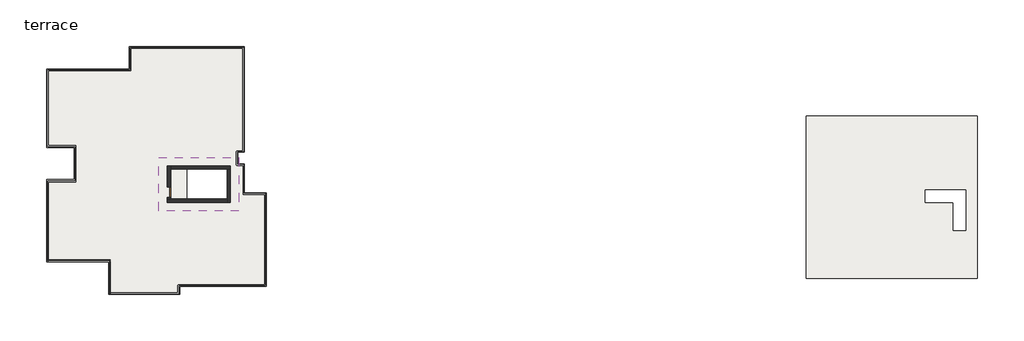
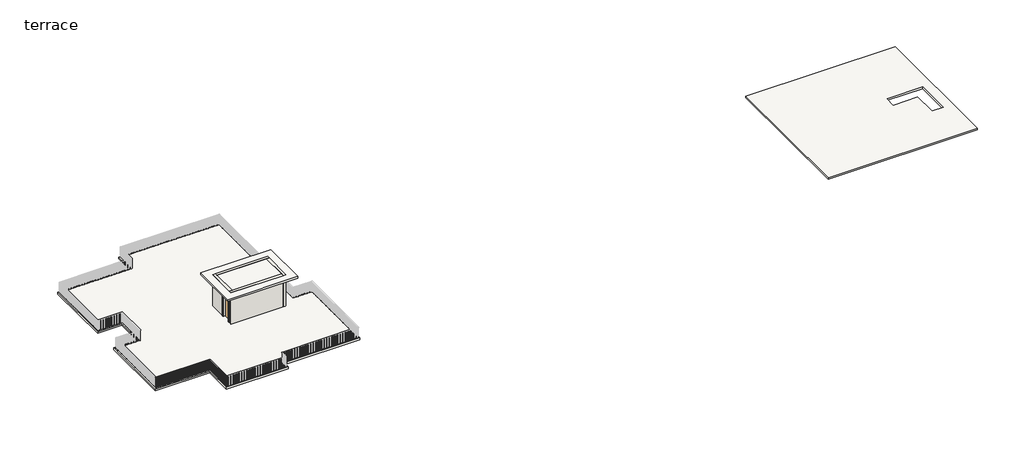
# One storey, part 1 of 7: 4 walls, 3 slabs, 2 railings, 1 door.
"""IFC4 building model written with IfcOpenShell, lengths in millimetres."""

from ifc_helpers import new_model, si_unit, frame, origin, place, context, project, spatial, polyline, outline, extrude, faceted_brep, transform, mapped, element, save
from components import door_bb98abfd

model = new_model("IFC4")

# Units and contexts
model_context = context("Model", 3, world=origin())
ifc_project = project(units=[si_unit("LENGTHUNIT", "METRE", prefix="MILLI")], contexts=[model_context])

# Site, building, storey
site = spatial("IfcSite", under=ifc_project)
building = spatial("IfcBuilding", under=site)
storey = spatial("IfcBuildingStorey", under=building, Name="terrace", Elevation=3810.0)

# Door
placement = place(None, origin())
door_shape = door_bb98abfd(model_context)
element("IfcDoor", 1, ObjectType="Single-Flush : 30\" x 84\"", at=placement, inside=storey, context=model_context, shape_type="MappedRepresentation", body=[
    mapped(door_shape, transform((-5641.4918815, 2189.5168074, 3810.0), x_axis=(0.0, -1.0, 0.0), y_axis=(1.0, 0.0, 0.0), z_axis=(0.0, 0.0, 1.0))),
])

# Railings
element("IfcRailing", 2, ObjectType="Handrail - Rectangular", at=placement, inside=storey, context=model_context, shape_type="SweptSolid", body=[
    extrude(outline(polyline([(-9876.7390129, -5140.022378), (-9927.5390129, -5140.022378), (-9927.5390129, -2803.222378), (-9876.7390129, -2803.222378), (-9876.7390129, -5140.022378)])), frame((0.0, 0.0, 4673.6), z_axis=(0.0, 0.0, 1.0), x_axis=(1.0, 0.0, 0.0)), (0.0, 0.0, 1.0), 50.8),
    extrude(outline(polyline([(-9892.6140129, -2914.347378), (-9911.6640129, -2914.347378), (-9911.6640129, -2895.297378), (-9892.6140129, -2895.297378), (-9892.6140129, -2914.347378)])), frame((0.0, 0.0, 3810.0), z_axis=(0.0, 0.0, 1.0), x_axis=(1.0, 0.0, 0.0)), (0.0, 0.0, 1.0), 863.6),
    extrude(outline(polyline([(-9892.6140129, -3015.947378), (-9911.6640129, -3015.947378), (-9911.6640129, -2996.897378), (-9892.6140129, -2996.897378), (-9892.6140129, -3015.947378)])), frame((0.0, 0.0, 3810.0), z_axis=(0.0, 0.0, 1.0), x_axis=(1.0, 0.0, 0.0)), (0.0, 0.0, 1.0), 863.6),
    extrude(outline(polyline([(-9892.6140129, -3117.547378), (-9911.6640129, -3117.547378), (-9911.6640129, -3098.497378), (-9892.6140129, -3098.497378), (-9892.6140129, -3117.547378)])), frame((0.0, 0.0, 3810.0), z_axis=(0.0, 0.0, 1.0), x_axis=(1.0, 0.0, 0.0)), (0.0, 0.0, 1.0), 863.6),
    extrude(outline(polyline([(-9892.6140129, -3219.147378), (-9911.6640129, -3219.147378), (-9911.6640129, -3200.097378), (-9892.6140129, -3200.097378), (-9892.6140129, -3219.147378)])), frame((0.0, 0.0, 3810.0), z_axis=(0.0, 0.0, 1.0), x_axis=(1.0, 0.0, 0.0)), (0.0, 0.0, 1.0), 863.6),
    extrude(outline(polyline([(-9892.6140129, -3320.747378), (-9911.6640129, -3320.747378), (-9911.6640129, -3301.697378), (-9892.6140129, -3301.697378), (-9892.6140129, -3320.747378)])), frame((0.0, 0.0, 3810.0), z_axis=(0.0, 0.0, 1.0), x_axis=(1.0, 0.0, 0.0)), (0.0, 0.0, 1.0), 863.6),
    extrude(outline(polyline([(-9892.6140129, -3422.347378), (-9911.6640129, -3422.347378), (-9911.6640129, -3403.297378), (-9892.6140129, -3403.297378), (-9892.6140129, -3422.347378)])), frame((0.0, 0.0, 3810.0), z_axis=(0.0, 0.0, 1.0), x_axis=(1.0, 0.0, 0.0)), (0.0, 0.0, 1.0), 863.6),
    extrude(outline(polyline([(-9892.6140129, -3523.947378), (-9911.6640129, -3523.947378), (-9911.6640129, -3504.897378), (-9892.6140129, -3504.897378), (-9892.6140129, -3523.947378)])), frame((0.0, 0.0, 3810.0), z_axis=(0.0, 0.0, 1.0), x_axis=(1.0, 0.0, 0.0)), (0.0, 0.0, 1.0), 863.6),
    extrude(outline(polyline([(-9892.6140129, -3625.547378), (-9911.6640129, -3625.547378), (-9911.6640129, -3606.497378), (-9892.6140129, -3606.497378), (-9892.6140129, -3625.547378)])), frame((0.0, 0.0, 3810.0), z_axis=(0.0, 0.0, 1.0), x_axis=(1.0, 0.0, 0.0)), (0.0, 0.0, 1.0), 863.6),
    extrude(outline(polyline([(-9892.6140129, -3727.147378), (-9911.6640129, -3727.147378), (-9911.6640129, -3708.097378), (-9892.6140129, -3708.097378), (-9892.6140129, -3727.147378)])), frame((0.0, 0.0, 3810.0), z_axis=(0.0, 0.0, 1.0), x_axis=(1.0, 0.0, 0.0)), (0.0, 0.0, 1.0), 863.6),
    extrude(outline(polyline([(-9892.6140129, -3828.747378), (-9911.6640129, -3828.747378), (-9911.6640129, -3809.697378), (-9892.6140129, -3809.697378), (-9892.6140129, -3828.747378)])), frame((0.0, 0.0, 3810.0), z_axis=(0.0, 0.0, 1.0), x_axis=(1.0, 0.0, 0.0)), (0.0, 0.0, 1.0), 863.6),
    extrude(outline(polyline([(-9892.6140129, -3930.347378), (-9911.6640129, -3930.347378), (-9911.6640129, -3911.297378), (-9892.6140129, -3911.297378), (-9892.6140129, -3930.347378)])), frame((0.0, 0.0, 3810.0), z_axis=(0.0, 0.0, 1.0), x_axis=(1.0, 0.0, 0.0)), (0.0, 0.0, 1.0), 863.6),
    extrude(outline(polyline([(-9892.6140129, -4031.947378), (-9911.6640129, -4031.947378), (-9911.6640129, -4012.897378), (-9892.6140129, -4012.897378), (-9892.6140129, -4031.947378)])), frame((0.0, 0.0, 3810.0), z_axis=(0.0, 0.0, 1.0), x_axis=(1.0, 0.0, 0.0)), (0.0, 0.0, 1.0), 863.6),
    extrude(outline(polyline([(-9892.6140129, -4133.547378), (-9911.6640129, -4133.547378), (-9911.6640129, -4114.497378), (-9892.6140129, -4114.497378), (-9892.6140129, -4133.547378)])), frame((0.0, 0.0, 3810.0), z_axis=(0.0, 0.0, 1.0), x_axis=(1.0, 0.0, 0.0)), (0.0, 0.0, 1.0), 863.6),
    extrude(outline(polyline([(-9892.6140129, -4235.147378), (-9911.6640129, -4235.147378), (-9911.6640129, -4216.097378), (-9892.6140129, -4216.097378), (-9892.6140129, -4235.147378)])), frame((0.0, 0.0, 3810.0), z_axis=(0.0, 0.0, 1.0), x_axis=(1.0, 0.0, 0.0)), (0.0, 0.0, 1.0), 863.6),
    extrude(outline(polyline([(-9892.6140129, -4336.747378), (-9911.6640129, -4336.747378), (-9911.6640129, -4317.697378), (-9892.6140129, -4317.697378), (-9892.6140129, -4336.747378)])), frame((0.0, 0.0, 3810.0), z_axis=(0.0, 0.0, 1.0), x_axis=(1.0, 0.0, 0.0)), (0.0, 0.0, 1.0), 863.6),
    extrude(outline(polyline([(-9892.6140129, -4438.347378), (-9911.6640129, -4438.347378), (-9911.6640129, -4419.297378), (-9892.6140129, -4419.297378), (-9892.6140129, -4438.347378)])), frame((0.0, 0.0, 3810.0), z_axis=(0.0, 0.0, 1.0), x_axis=(1.0, 0.0, 0.0)), (0.0, 0.0, 1.0), 863.6),
    extrude(outline(polyline([(-9892.6140129, -4539.947378), (-9911.6640129, -4539.947378), (-9911.6640129, -4520.897378), (-9892.6140129, -4520.897378), (-9892.6140129, -4539.947378)])), frame((0.0, 0.0, 3810.0), z_axis=(0.0, 0.0, 1.0), x_axis=(1.0, 0.0, 0.0)), (0.0, 0.0, 1.0), 863.6),
    extrude(outline(polyline([(-9892.6140129, -4641.547378), (-9911.6640129, -4641.547378), (-9911.6640129, -4622.497378), (-9892.6140129, -4622.497378), (-9892.6140129, -4641.547378)])), frame((0.0, 0.0, 3810.0), z_axis=(0.0, 0.0, 1.0), x_axis=(1.0, 0.0, 0.0)), (0.0, 0.0, 1.0), 863.6),
    extrude(outline(polyline([(-9892.6140129, -4743.147378), (-9911.6640129, -4743.147378), (-9911.6640129, -4724.097378), (-9892.6140129, -4724.097378), (-9892.6140129, -4743.147378)])), frame((0.0, 0.0, 3810.0), z_axis=(0.0, 0.0, 1.0), x_axis=(1.0, 0.0, 0.0)), (0.0, 0.0, 1.0), 863.6),
    extrude(outline(polyline([(-9892.6140129, -4844.747378), (-9911.6640129, -4844.747378), (-9911.6640129, -4825.697378), (-9892.6140129, -4825.697378), (-9892.6140129, -4844.747378)])), frame((0.0, 0.0, 3810.0), z_axis=(0.0, 0.0, 1.0), x_axis=(1.0, 0.0, 0.0)), (0.0, 0.0, 1.0), 863.6),
    extrude(outline(polyline([(-9892.6140129, -4946.347378), (-9911.6640129, -4946.347378), (-9911.6640129, -4927.297378), (-9892.6140129, -4927.297378), (-9892.6140129, -4946.347378)])), frame((0.0, 0.0, 3810.0), z_axis=(0.0, 0.0, 1.0), x_axis=(1.0, 0.0, 0.0)), (0.0, 0.0, 1.0), 863.6),
    extrude(outline(polyline([(-9892.6140129, -5047.947378), (-9911.6640129, -5047.947378), (-9911.6640129, -5028.897378), (-9892.6140129, -5028.897378), (-9892.6140129, -5047.947378)])), frame((0.0, 0.0, 3810.0), z_axis=(0.0, 0.0, 1.0), x_axis=(1.0, 0.0, 0.0)), (0.0, 0.0, 1.0), 863.6),
    extrude(outline(polyline([(-9892.6140129, -2822.272378), (-9911.6640129, -2822.272378), (-9911.6640129, -2803.222378), (-9892.6140129, -2803.222378), (-9892.6140129, -2822.272378)])), frame((0.0, 0.0, 3810.0), z_axis=(0.0, 0.0, 1.0), x_axis=(1.0, 0.0, 0.0)), (0.0, 0.0, 1.0), 863.6),
    extrude(outline(polyline([(-9892.6140129, -5140.022378), (-9911.6640129, -5140.022378), (-9911.6640129, -5120.972378), (-9892.6140129, -5120.972378), (-9892.6140129, -5140.022378)])), frame((0.0, 0.0, 3810.0), z_axis=(0.0, 0.0, 1.0), x_axis=(1.0, 0.0, 0.0)), (0.0, 0.0, 1.0), 863.6),
])
element("IfcRailing", 3, ObjectType="Handrail - Rectangular", at=placement, inside=storey, context=model_context, shape_type="SweptSolid", body=[
    extrude(outline(polyline([(-9895.7890129, -2701.622378), (-9895.7890129, -2752.422378), (-14391.5890129, -2752.422378), (-14391.5890129, -2701.622378), (-9895.7890129, -2701.622378)])), frame((0.0, 0.0, 4673.6), z_axis=(0.0, 0.0, 1.0), x_axis=(1.0, 0.0, 0.0)), (0.0, 0.0, 1.0), 50.8),
    extrude(outline(polyline([(-14356.6640129, -2717.497378), (-14356.6640129, -2736.547378), (-14375.7140129, -2736.547378), (-14375.7140129, -2717.497378), (-14356.6640129, -2717.497378)])), frame((0.0, 0.0, 3810.0), z_axis=(0.0, 0.0, 1.0), x_axis=(1.0, 0.0, 0.0)), (0.0, 0.0, 1.0), 863.6),
    extrude(outline(polyline([(-14255.0640129, -2717.497378), (-14255.0640129, -2736.547378), (-14274.1140129, -2736.547378), (-14274.1140129, -2717.497378), (-14255.0640129, -2717.497378)])), frame((0.0, 0.0, 3810.0), z_axis=(0.0, 0.0, 1.0), x_axis=(1.0, 0.0, 0.0)), (0.0, 0.0, 1.0), 863.6),
    extrude(outline(polyline([(-14153.4640129, -2717.497378), (-14153.4640129, -2736.547378), (-14172.5140129, -2736.547378), (-14172.5140129, -2717.497378), (-14153.4640129, -2717.497378)])), frame((0.0, 0.0, 3810.0), z_axis=(0.0, 0.0, 1.0), x_axis=(1.0, 0.0, 0.0)), (0.0, 0.0, 1.0), 863.6),
    extrude(outline(polyline([(-14051.8640129, -2717.497378), (-14051.8640129, -2736.547378), (-14070.9140129, -2736.547378), (-14070.9140129, -2717.497378), (-14051.8640129, -2717.497378)])), frame((0.0, 0.0, 3810.0), z_axis=(0.0, 0.0, 1.0), x_axis=(1.0, 0.0, 0.0)), (0.0, 0.0, 1.0), 863.6),
    extrude(outline(polyline([(-13950.2640129, -2717.497378), (-13950.2640129, -2736.547378), (-13969.3140129, -2736.547378), (-13969.3140129, -2717.497378), (-13950.2640129, -2717.497378)])), frame((0.0, 0.0, 3810.0), z_axis=(0.0, 0.0, 1.0), x_axis=(1.0, 0.0, 0.0)), (0.0, 0.0, 1.0), 863.6),
    extrude(outline(polyline([(-13848.6640129, -2717.497378), (-13848.6640129, -2736.547378), (-13867.7140129, -2736.547378), (-13867.7140129, -2717.497378), (-13848.6640129, -2717.497378)])), frame((0.0, 0.0, 3810.0), z_axis=(0.0, 0.0, 1.0), x_axis=(1.0, 0.0, 0.0)), (0.0, 0.0, 1.0), 863.6),
    extrude(outline(polyline([(-13747.0640129, -2717.497378), (-13747.0640129, -2736.547378), (-13766.1140129, -2736.547378), (-13766.1140129, -2717.497378), (-13747.0640129, -2717.497378)])), frame((0.0, 0.0, 3810.0), z_axis=(0.0, 0.0, 1.0), x_axis=(1.0, 0.0, 0.0)), (0.0, 0.0, 1.0), 863.6),
    extrude(outline(polyline([(-13645.4640129, -2717.497378), (-13645.4640129, -2736.547378), (-13664.5140129, -2736.547378), (-13664.5140129, -2717.497378), (-13645.4640129, -2717.497378)])), frame((0.0, 0.0, 3810.0), z_axis=(0.0, 0.0, 1.0), x_axis=(1.0, 0.0, 0.0)), (0.0, 0.0, 1.0), 863.6),
    extrude(outline(polyline([(-13543.8640129, -2717.497378), (-13543.8640129, -2736.547378), (-13562.9140129, -2736.547378), (-13562.9140129, -2717.497378), (-13543.8640129, -2717.497378)])), frame((0.0, 0.0, 3810.0), z_axis=(0.0, 0.0, 1.0), x_axis=(1.0, 0.0, 0.0)), (0.0, 0.0, 1.0), 863.6),
    extrude(outline(polyline([(-13442.2640129, -2717.497378), (-13442.2640129, -2736.547378), (-13461.3140129, -2736.547378), (-13461.3140129, -2717.497378), (-13442.2640129, -2717.497378)])), frame((0.0, 0.0, 3810.0), z_axis=(0.0, 0.0, 1.0), x_axis=(1.0, 0.0, 0.0)), (0.0, 0.0, 1.0), 863.6),
    extrude(outline(polyline([(-13340.6640129, -2717.497378), (-13340.6640129, -2736.547378), (-13359.7140129, -2736.547378), (-13359.7140129, -2717.497378), (-13340.6640129, -2717.497378)])), frame((0.0, 0.0, 3810.0), z_axis=(0.0, 0.0, 1.0), x_axis=(1.0, 0.0, 0.0)), (0.0, 0.0, 1.0), 863.6),
    extrude(outline(polyline([(-13239.0640129, -2717.497378), (-13239.0640129, -2736.547378), (-13258.1140129, -2736.547378), (-13258.1140129, -2717.497378), (-13239.0640129, -2717.497378)])), frame((0.0, 0.0, 3810.0), z_axis=(0.0, 0.0, 1.0), x_axis=(1.0, 0.0, 0.0)), (0.0, 0.0, 1.0), 863.6),
    extrude(outline(polyline([(-13137.4640129, -2717.497378), (-13137.4640129, -2736.547378), (-13156.5140129, -2736.547378), (-13156.5140129, -2717.497378), (-13137.4640129, -2717.497378)])), frame((0.0, 0.0, 3810.0), z_axis=(0.0, 0.0, 1.0), x_axis=(1.0, 0.0, 0.0)), (0.0, 0.0, 1.0), 863.6),
    extrude(outline(polyline([(-13035.8640129, -2717.497378), (-13035.8640129, -2736.547378), (-13054.9140129, -2736.547378), (-13054.9140129, -2717.497378), (-13035.8640129, -2717.497378)])), frame((0.0, 0.0, 3810.0), z_axis=(0.0, 0.0, 1.0), x_axis=(1.0, 0.0, 0.0)), (0.0, 0.0, 1.0), 863.6),
    extrude(outline(polyline([(-12934.2640129, -2717.497378), (-12934.2640129, -2736.547378), (-12953.3140129, -2736.547378), (-12953.3140129, -2717.497378), (-12934.2640129, -2717.497378)])), frame((0.0, 0.0, 3810.0), z_axis=(0.0, 0.0, 1.0), x_axis=(1.0, 0.0, 0.0)), (0.0, 0.0, 1.0), 863.6),
    extrude(outline(polyline([(-12832.6640129, -2717.497378), (-12832.6640129, -2736.547378), (-12851.7140129, -2736.547378), (-12851.7140129, -2717.497378), (-12832.6640129, -2717.497378)])), frame((0.0, 0.0, 3810.0), z_axis=(0.0, 0.0, 1.0), x_axis=(1.0, 0.0, 0.0)), (0.0, 0.0, 1.0), 863.6),
    extrude(outline(polyline([(-12731.0640129, -2717.497378), (-12731.0640129, -2736.547378), (-12750.1140129, -2736.547378), (-12750.1140129, -2717.497378), (-12731.0640129, -2717.497378)])), frame((0.0, 0.0, 3810.0), z_axis=(0.0, 0.0, 1.0), x_axis=(1.0, 0.0, 0.0)), (0.0, 0.0, 1.0), 863.6),
    extrude(outline(polyline([(-12629.4640129, -2717.497378), (-12629.4640129, -2736.547378), (-12648.5140129, -2736.547378), (-12648.5140129, -2717.497378), (-12629.4640129, -2717.497378)])), frame((0.0, 0.0, 3810.0), z_axis=(0.0, 0.0, 1.0), x_axis=(1.0, 0.0, 0.0)), (0.0, 0.0, 1.0), 863.6),
    extrude(outline(polyline([(-12527.8640129, -2717.497378), (-12527.8640129, -2736.547378), (-12546.9140129, -2736.547378), (-12546.9140129, -2717.497378), (-12527.8640129, -2717.497378)])), frame((0.0, 0.0, 3810.0), z_axis=(0.0, 0.0, 1.0), x_axis=(1.0, 0.0, 0.0)), (0.0, 0.0, 1.0), 863.6),
    extrude(outline(polyline([(-12426.2640129, -2717.497378), (-12426.2640129, -2736.547378), (-12445.3140129, -2736.547378), (-12445.3140129, -2717.497378), (-12426.2640129, -2717.497378)])), frame((0.0, 0.0, 3810.0), z_axis=(0.0, 0.0, 1.0), x_axis=(1.0, 0.0, 0.0)), (0.0, 0.0, 1.0), 863.6),
    extrude(outline(polyline([(-12324.6640129, -2717.497378), (-12324.6640129, -2736.547378), (-12343.7140129, -2736.547378), (-12343.7140129, -2717.497378), (-12324.6640129, -2717.497378)])), frame((0.0, 0.0, 3810.0), z_axis=(0.0, 0.0, 1.0), x_axis=(1.0, 0.0, 0.0)), (0.0, 0.0, 1.0), 863.6),
    extrude(outline(polyline([(-12223.0640129, -2717.497378), (-12223.0640129, -2736.547378), (-12242.1140129, -2736.547378), (-12242.1140129, -2717.497378), (-12223.0640129, -2717.497378)])), frame((0.0, 0.0, 3810.0), z_axis=(0.0, 0.0, 1.0), x_axis=(1.0, 0.0, 0.0)), (0.0, 0.0, 1.0), 863.6),
    extrude(outline(polyline([(-12121.4640129, -2717.497378), (-12121.4640129, -2736.547378), (-12140.5140129, -2736.547378), (-12140.5140129, -2717.497378), (-12121.4640129, -2717.497378)])), frame((0.0, 0.0, 3810.0), z_axis=(0.0, 0.0, 1.0), x_axis=(1.0, 0.0, 0.0)), (0.0, 0.0, 1.0), 863.6),
    extrude(outline(polyline([(-12019.8640129, -2717.497378), (-12019.8640129, -2736.547378), (-12038.9140129, -2736.547378), (-12038.9140129, -2717.497378), (-12019.8640129, -2717.497378)])), frame((0.0, 0.0, 3810.0), z_axis=(0.0, 0.0, 1.0), x_axis=(1.0, 0.0, 0.0)), (0.0, 0.0, 1.0), 863.6),
    extrude(outline(polyline([(-11918.2640129, -2717.497378), (-11918.2640129, -2736.547378), (-11937.3140129, -2736.547378), (-11937.3140129, -2717.497378), (-11918.2640129, -2717.497378)])), frame((0.0, 0.0, 3810.0), z_axis=(0.0, 0.0, 1.0), x_axis=(1.0, 0.0, 0.0)), (0.0, 0.0, 1.0), 863.6),
    extrude(outline(polyline([(-11816.6640129, -2717.497378), (-11816.6640129, -2736.547378), (-11835.7140129, -2736.547378), (-11835.7140129, -2717.497378), (-11816.6640129, -2717.497378)])), frame((0.0, 0.0, 3810.0), z_axis=(0.0, 0.0, 1.0), x_axis=(1.0, 0.0, 0.0)), (0.0, 0.0, 1.0), 863.6),
    extrude(outline(polyline([(-11715.0640129, -2717.497378), (-11715.0640129, -2736.547378), (-11734.1140129, -2736.547378), (-11734.1140129, -2717.497378), (-11715.0640129, -2717.497378)])), frame((0.0, 0.0, 3810.0), z_axis=(0.0, 0.0, 1.0), x_axis=(1.0, 0.0, 0.0)), (0.0, 0.0, 1.0), 863.6),
    extrude(outline(polyline([(-11613.4640129, -2717.497378), (-11613.4640129, -2736.547378), (-11632.5140129, -2736.547378), (-11632.5140129, -2717.497378), (-11613.4640129, -2717.497378)])), frame((0.0, 0.0, 3810.0), z_axis=(0.0, 0.0, 1.0), x_axis=(1.0, 0.0, 0.0)), (0.0, 0.0, 1.0), 863.6),
    extrude(outline(polyline([(-11511.8640129, -2717.497378), (-11511.8640129, -2736.547378), (-11530.9140129, -2736.547378), (-11530.9140129, -2717.497378), (-11511.8640129, -2717.497378)])), frame((0.0, 0.0, 3810.0), z_axis=(0.0, 0.0, 1.0), x_axis=(1.0, 0.0, 0.0)), (0.0, 0.0, 1.0), 863.6),
    extrude(outline(polyline([(-11410.2640129, -2717.497378), (-11410.2640129, -2736.547378), (-11429.3140129, -2736.547378), (-11429.3140129, -2717.497378), (-11410.2640129, -2717.497378)])), frame((0.0, 0.0, 3810.0), z_axis=(0.0, 0.0, 1.0), x_axis=(1.0, 0.0, 0.0)), (0.0, 0.0, 1.0), 863.6),
    extrude(outline(polyline([(-11308.6640129, -2717.497378), (-11308.6640129, -2736.547378), (-11327.7140129, -2736.547378), (-11327.7140129, -2717.497378), (-11308.6640129, -2717.497378)])), frame((0.0, 0.0, 3810.0), z_axis=(0.0, 0.0, 1.0), x_axis=(1.0, 0.0, 0.0)), (0.0, 0.0, 1.0), 863.6),
    extrude(outline(polyline([(-11207.0640129, -2717.497378), (-11207.0640129, -2736.547378), (-11226.1140129, -2736.547378), (-11226.1140129, -2717.497378), (-11207.0640129, -2717.497378)])), frame((0.0, 0.0, 3810.0), z_axis=(0.0, 0.0, 1.0), x_axis=(1.0, 0.0, 0.0)), (0.0, 0.0, 1.0), 863.6),
    extrude(outline(polyline([(-11105.4640129, -2717.497378), (-11105.4640129, -2736.547378), (-11124.5140129, -2736.547378), (-11124.5140129, -2717.497378), (-11105.4640129, -2717.497378)])), frame((0.0, 0.0, 3810.0), z_axis=(0.0, 0.0, 1.0), x_axis=(1.0, 0.0, 0.0)), (0.0, 0.0, 1.0), 863.6),
    extrude(outline(polyline([(-11003.8640129, -2717.497378), (-11003.8640129, -2736.547378), (-11022.9140129, -2736.547378), (-11022.9140129, -2717.497378), (-11003.8640129, -2717.497378)])), frame((0.0, 0.0, 3810.0), z_axis=(0.0, 0.0, 1.0), x_axis=(1.0, 0.0, 0.0)), (0.0, 0.0, 1.0), 863.6),
    extrude(outline(polyline([(-10902.2640129, -2717.497378), (-10902.2640129, -2736.547378), (-10921.3140129, -2736.547378), (-10921.3140129, -2717.497378), (-10902.2640129, -2717.497378)])), frame((0.0, 0.0, 3810.0), z_axis=(0.0, 0.0, 1.0), x_axis=(1.0, 0.0, 0.0)), (0.0, 0.0, 1.0), 863.6),
    extrude(outline(polyline([(-10800.6640129, -2717.497378), (-10800.6640129, -2736.547378), (-10819.7140129, -2736.547378), (-10819.7140129, -2717.497378), (-10800.6640129, -2717.497378)])), frame((0.0, 0.0, 3810.0), z_axis=(0.0, 0.0, 1.0), x_axis=(1.0, 0.0, 0.0)), (0.0, 0.0, 1.0), 863.6),
    extrude(outline(polyline([(-10699.0640129, -2717.497378), (-10699.0640129, -2736.547378), (-10718.1140129, -2736.547378), (-10718.1140129, -2717.497378), (-10699.0640129, -2717.497378)])), frame((0.0, 0.0, 3810.0), z_axis=(0.0, 0.0, 1.0), x_axis=(1.0, 0.0, 0.0)), (0.0, 0.0, 1.0), 863.6),
    extrude(outline(polyline([(-10597.4640129, -2717.497378), (-10597.4640129, -2736.547378), (-10616.5140129, -2736.547378), (-10616.5140129, -2717.497378), (-10597.4640129, -2717.497378)])), frame((0.0, 0.0, 3810.0), z_axis=(0.0, 0.0, 1.0), x_axis=(1.0, 0.0, 0.0)), (0.0, 0.0, 1.0), 863.6),
    extrude(outline(polyline([(-10495.8640129, -2717.497378), (-10495.8640129, -2736.547378), (-10514.9140129, -2736.547378), (-10514.9140129, -2717.497378), (-10495.8640129, -2717.497378)])), frame((0.0, 0.0, 3810.0), z_axis=(0.0, 0.0, 1.0), x_axis=(1.0, 0.0, 0.0)), (0.0, 0.0, 1.0), 863.6),
    extrude(outline(polyline([(-10394.2640129, -2717.497378), (-10394.2640129, -2736.547378), (-10413.3140129, -2736.547378), (-10413.3140129, -2717.497378), (-10394.2640129, -2717.497378)])), frame((0.0, 0.0, 3810.0), z_axis=(0.0, 0.0, 1.0), x_axis=(1.0, 0.0, 0.0)), (0.0, 0.0, 1.0), 863.6),
    extrude(outline(polyline([(-10292.6640129, -2717.497378), (-10292.6640129, -2736.547378), (-10311.7140129, -2736.547378), (-10311.7140129, -2717.497378), (-10292.6640129, -2717.497378)])), frame((0.0, 0.0, 3810.0), z_axis=(0.0, 0.0, 1.0), x_axis=(1.0, 0.0, 0.0)), (0.0, 0.0, 1.0), 863.6),
    extrude(outline(polyline([(-10191.0640129, -2717.497378), (-10191.0640129, -2736.547378), (-10210.1140129, -2736.547378), (-10210.1140129, -2717.497378), (-10191.0640129, -2717.497378)])), frame((0.0, 0.0, 3810.0), z_axis=(0.0, 0.0, 1.0), x_axis=(1.0, 0.0, 0.0)), (0.0, 0.0, 1.0), 863.6),
    extrude(outline(polyline([(-10089.4640129, -2717.497378), (-10089.4640129, -2736.547378), (-10108.5140129, -2736.547378), (-10108.5140129, -2717.497378), (-10089.4640129, -2717.497378)])), frame((0.0, 0.0, 3810.0), z_axis=(0.0, 0.0, 1.0), x_axis=(1.0, 0.0, 0.0)), (0.0, 0.0, 1.0), 863.6),
    extrude(outline(polyline([(-9987.8640129, -2717.497378), (-9987.8640129, -2736.547378), (-10006.9140129, -2736.547378), (-10006.9140129, -2717.497378), (-9987.8640129, -2717.497378)])), frame((0.0, 0.0, 3810.0), z_axis=(0.0, 0.0, 1.0), x_axis=(1.0, 0.0, 0.0)), (0.0, 0.0, 1.0), 863.6),
    extrude(outline(polyline([(-14372.5390129, -2717.497378), (-14372.5390129, -2736.547378), (-14391.5890129, -2736.547378), (-14391.5890129, -2717.497378), (-14372.5390129, -2717.497378)])), frame((0.0, 0.0, 3810.0), z_axis=(0.0, 0.0, 1.0), x_axis=(1.0, 0.0, 0.0)), (0.0, 0.0, 1.0), 863.6),
    extrude(outline(polyline([(-9895.7890129, -2717.497378), (-9895.7890129, -2736.547378), (-9914.8390129, -2736.547378), (-9914.8390129, -2717.497378), (-9895.7890129, -2717.497378)])), frame((0.0, 0.0, 3810.0), z_axis=(0.0, 0.0, 1.0), x_axis=(1.0, 0.0, 0.0)), (0.0, 0.0, 1.0), 863.6),
])

# Slabs
element("IfcSlab", 4, ObjectType="Generic - 2\" 9", at=placement, inside=storey, context=model_context, shape_type="SweptSolid", body=[
    extrude(outline(polyline([(52729.9357782, 7692.1642693), (52729.9357782, -4042.6357307), (40385.5357782, -4042.6357307), (40385.5357782, 7692.1642693), (52729.9357782, 7692.1642693)]), holes=[polyline([(51891.7357782, 2358.1642693), (48955.7987887, 2358.1642693), (48955.7987887, 1443.7642693), (50977.3357782, 1443.7642693), (50977.3357782, -577.7727202), (51891.7357782, -577.7727202), (51891.7357782, 2358.1642693)])]), frame((0.0, 0.0, 3657.6), z_axis=(0.0, 0.0, 1.0), x_axis=(1.0, 0.0, 0.0)), (0.0, 0.0, 1.0), 152.4),
])
element("IfcSlab", 5, ObjectType="Generic - 6\" 3", at=placement, inside=storey, context=model_context, shape_type="SweptSolid", body=[
    extrude(outline(polyline([(-8499.7719122, 11092.2168074), (-8499.7719122, 12730.5168074), (-193.9719122, 12730.5168074), (-193.9719122, 5091.4668074), (-689.2719122, 5091.4668074), (-689.2719122, 4215.1668074), (-193.9719122, 4215.1668074), (-193.9719122, 2148.2418074), (1374.4780878, 2148.2418074), (1374.4780878, -4614.5081926), (-4879.4781622, -4614.5081926), (-4879.4781622, -5195.5331926), (-9985.6719122, -5195.5331926), (-9985.6719122, -2852.3831926), (-14481.4719122, -2852.3831926), (-14481.4719122, 3110.2668074), (-12481.2219122, 3110.2668074), (-12481.2219122, 5434.3668074), (-14481.4719122, 5434.3668074), (-14481.4719122, 11092.2168074), (-8499.7719122, 11092.2168074)]), holes=[polyline([(-1437.7918815, 3859.5668074), (-4333.3918815, 3859.5668074), (-4333.3918815, 1694.2168074), (-1437.7918815, 1694.2168074), (-1437.7918815, 3859.5668074)])]), frame((0.0, 0.0, 3657.6), z_axis=(0.0, 0.0, 1.0), x_axis=(1.0, 0.0, 0.0)), (0.0, 0.0, 1.0), 152.4),
])
element("IfcSlab", 6, ObjectType="Generic - 6\" 5", at=placement, inside=storey, context=model_context, shape_type="SweptSolid", body=[
    extrude(outline(polyline([(-599.5918815, 4697.7668074), (-599.5918815, 856.0168074), (-6365.3918815, 856.0168074), (-6365.3918815, 4697.7668074), (-599.5918815, 4697.7668074)])), frame((0.0, 0.0, 6400.8), z_axis=(0.0, 0.0, 1.0), x_axis=(1.0, 0.0, 0.0)), (0.0, 0.0, 1.0), 152.4),
])

# Walls
element("IfcWall", 7, ObjectType="Generic - 9\"", at=placement, inside=storey, context=model_context, shape_type="Brep", body=[
    faceted_brep([(-5527.1918815, 3859.5668074, 3810.0), (-1437.7918815, 3859.5668074, 3810.0), (-1209.1918815, 3859.5668074, 3810.0), (-1209.1918815, 3859.5668074, 6553.2), (-1437.7918815, 3859.5668074, 6553.2), (-5527.1918815, 3859.5668074, 6553.2), (-5527.1918815, 4088.1668074, 3810.0), (-5527.1918815, 4088.1668074, 6553.2), (-1209.1918815, 4088.1668074, 6553.2), (-1209.1918815, 4088.1668074, 3810.0)], [[[0, 1, 2, 3, 4, 5]], [[6, 7, 8, 9]], [[2, 1, 0, 6, 9]], [[5, 4, 3, 8, 7]], [[3, 2, 9, 8]], [[0, 5, 7, 6]]]),
])
element("IfcWall", 8, ObjectType="Generic - 9\"", at=placement, inside=storey, context=model_context, shape_type="Brep", body=[
    faceted_brep([(-1437.7918815, 3859.5668074, 3810.0), (-1437.7918815, 1694.2168074, 3810.0), (-1437.7918815, 1465.6168074, 3810.0), (-1437.7918815, 1465.6168074, 6553.2), (-1437.7918815, 1694.2168074, 6553.2), (-1437.7918815, 3859.5668074, 6553.2), (-1209.1918815, 3859.5668074, 3810.0), (-1209.1918815, 3859.5668074, 6553.2), (-1209.1918815, 1465.6168074, 6553.2), (-1209.1918815, 1465.6168074, 3810.0)], [[[0, 1, 2, 3, 4, 5]], [[6, 7, 8, 9]], [[2, 1, 0, 6, 9]], [[5, 4, 3, 8, 7]], [[0, 5, 7, 6]], [[3, 2, 9, 8]]]),
])
element("IfcWall", 9, ObjectType="Generic - 9\"", at=placement, inside=storey, context=model_context, shape_type="Brep", body=[
    faceted_brep([(-1437.7918815, 1694.2168074, 3810.0), (-5527.1918815, 1694.2168074, 3810.0), (-5755.7918815, 1694.2168074, 3810.0), (-5755.7918815, 1694.2168074, 6553.2), (-5527.1918815, 1694.2168074, 6553.2), (-1437.7918815, 1694.2168074, 6553.2), (-1437.7918815, 1465.6168074, 3810.0), (-1437.7918815, 1465.6168074, 6553.2), (-5755.7918815, 1465.6168074, 6553.2), (-5755.7918815, 1465.6168074, 3810.0)], [[[0, 1, 2, 3, 4, 5]], [[6, 7, 8, 9]], [[2, 1, 0, 6, 9]], [[5, 4, 3, 8, 7]], [[0, 5, 7, 6]], [[3, 2, 9, 8]]]),
])
element("IfcWall", 10, ObjectType="Generic - 9\"", at=placement, inside=storey, context=model_context, shape_type="Brep", body=[
    faceted_brep([(-5527.1918815, 1694.2168074, 3810.0), (-5527.1918815, 1808.5168074, 3810.0), (-5527.1918815, 1808.5168074, 5943.6), (-5527.1918815, 2570.5168074, 5943.6), (-5527.1918815, 2570.5168074, 3810.0), (-5527.1918815, 3859.5668074, 3810.0), (-5527.1918815, 4088.1668074, 3810.0), (-5527.1918815, 4088.1668074, 6553.2), (-5527.1918815, 3859.5668074, 6553.2), (-5527.1918815, 1694.2168074, 6553.2), (-5755.7918815, 1808.5168074, 5943.6), (-5755.7918815, 1808.5168074, 3810.0), (-5755.7918815, 1694.2168074, 3810.0), (-5755.7918815, 1694.2168074, 6553.2), (-5755.7918815, 4088.1668074, 6553.2), (-5755.7918815, 4088.1668074, 3810.0), (-5755.7918815, 2570.5168074, 3810.0), (-5755.7918815, 2570.5168074, 5943.6)], [[[0, 1, 2, 3, 4, 5, 6, 7, 8, 9]], [[10, 11, 12, 13, 14, 15, 16, 17]], [[16, 15, 6, 5, 4]], [[12, 11, 1, 0]], [[9, 8, 7, 14, 13]], [[0, 9, 13, 12]], [[7, 6, 15, 14]], [[2, 1, 11, 10]], [[3, 2, 10, 17]], [[4, 3, 17, 16]]]),
])

save(model, "model.ifc")

# Revit data of these elements
# Type "Single-Flush : 30\" x 84\""
#   Type Mark = "4"
#   Construction Type Id = "MDOOR"
#   Assembly Code = "C1020"
#   Analytic Construction = "Metal"
#   Thickness = 0' - 2"
#   Heat Transfer Coefficient (U) = 0.651978 BTU/(h·ft²·°F)
#   Height = 7' - 0"
#   Trim Projection Ext = 0' - 1"
#   Trim Projection Int = 0' - 1"
#   Trim Width = 0' - 3"
#   Width = 2' - 6"
#   Define Thermal Properties by = 1
#   Define Thermal Properties by = 1
#   Door Material = Door - Panel
#   Frame Material = Door - Frame
#   Visual Light Transmittance = 0
#   Solar Heat Gain Coefficient = 0
#   Function = (empty or 0)
#   Wall Closure = (empty or 0)
# Type "Handrail - Rectangular"
#   Assembly Code = "C2010400"
#   built-in parameter 1008612 = 0.0416667 (stored number, unit not read)
#   built-in parameter 1008611 = 0.0416667 (stored number, unit not read)
#   built-in parameter 1008609 = 0.333333 (stored number, unit not read)
#   built-in parameter 1008604 = 0.166667 (stored number, unit not read)
#   built-in parameter 1008603 = 0.166667 (stored number, unit not read)
#   Railing Height = 3' - 0"
#   built-in parameter 1008630 = 2
#   built-in parameter 1008610 = 2
#   built-in parameter 1008618 = Baluster - Square : 3/4"
# Type "Generic - 2\" 9"
#   Assembly Code = "B1010"
#   Function = 0
#   Layers, outside or top first: 0' - 6" "Default" (function 1)
# Type "Generic - 6\" 3"
#   Assembly Code = "B1010"
#   Function = 0
#   Layers, outside or top first: 0' - 6" no material (function 1)
# Type "Generic - 6\" 5"
#   Assembly Code = "B1010"
#   Function = 0
#   Layers, outside or top first: 0' - 6" "Concrete, Cast-in-Place gray" (function 1)
# Type "Generic - 9\""
#   Assembly Code = "B2010"
#   Layers, outside or top first: 0' - 9" no material (function 1)
# Element 1 (IfcDoor, "Single-Flush : 30\" x 84\"")
#   Phase Created = New Construction
#   Materials on its faces: "Door - Frame", "Door - Panel"
# Elements 2, 3 (IfcRailing, "Handrail - Rectangular")
#   Phase Created = New Construction
# Element 4 (IfcSlab, "Generic - 2\" 9")
#   Height Offset From Level = 0' - 0"
#   Phase Created = New Construction
#   Materials on its faces: "Default"
# Element 5 (IfcSlab, "Generic - 6\" 3")
#   Height Offset From Level = 0' - 0"
#   Phase Created = New Construction
#   Materials on its faces: "Default Floor"
# Element 6 (IfcSlab, "Generic - 6\" 5")
#   Height Offset From Level = 9' - 0"
#   Phase Created = New Construction
#   Materials on its faces: "Concrete, Cast-in-Place gray"
# Elements 7, 8, 9, 10 (IfcWall, "Generic - 9\"")
#   Top Offset = 0' - 0"
#   Base Offset = 0' - 0"
#   Unconnected Height = 9' - 0"
#   wall height = 9' - 0"
#   Phase Created = New Construction
#   Base Constraint = terrace
#   Materials on its faces: "Default Wall"
# Materials
#   "Door - Panel": class "Wood", colour RGB 210 159 95, transparency 0, Cost = 0
#   "Door - Frame": colour RGB 118 70 51, transparency 0, Cost = 0
#   "Default": colour RGB 127 127 127, transparency 0, Cost = 0
#   "Concrete, Cast-in-Place gray": class "Concrete", colour RGB 192 192 192, transparency 0, Description = "Cast-in-place concrete", Cost = 0
#   "Default Floor": colour RGB 128 128 128, transparency 0, Cost = 0
#   "Default Wall": colour RGB 128 128 128, transparency 0, Cost = 0
